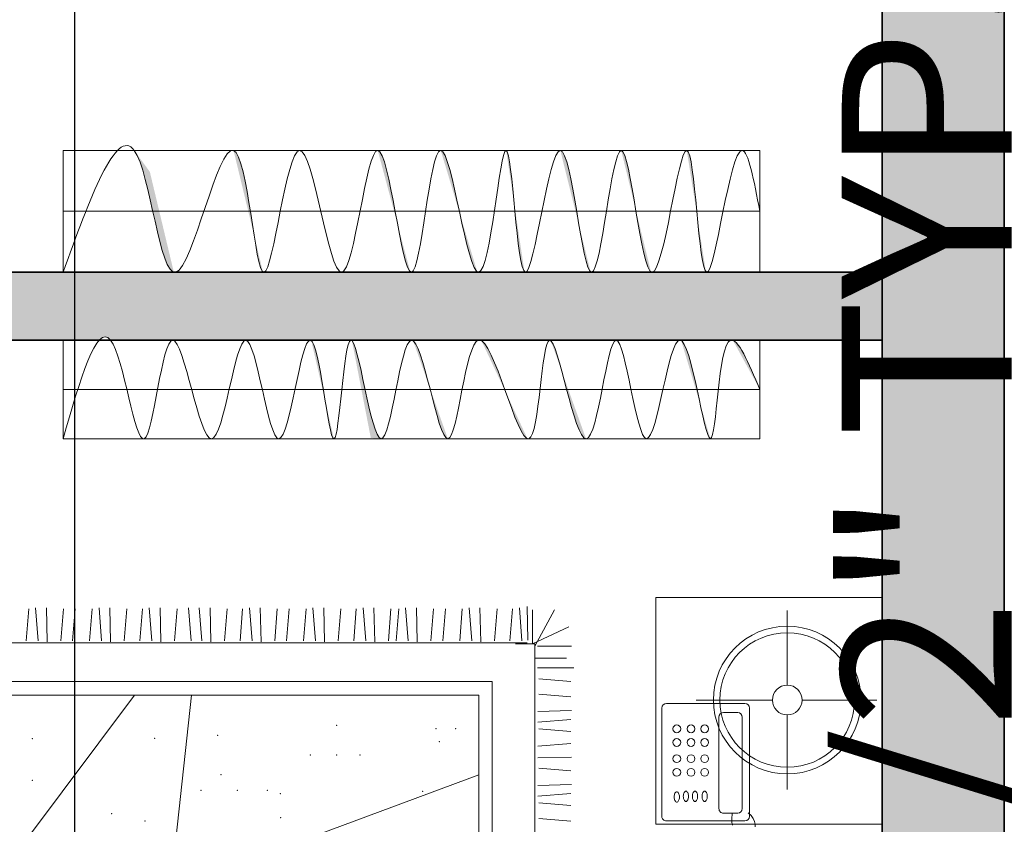
# Model space of a CAD drawing. Units: inches. Extents: x 1763 to 2368, y 1500 to 2097.
# Tile 15 of 24: x 2117 to 2189, y 1797 to 1856. Entities that reach past the tile are written whole.
import ezdxf

# ---------------------------------------------------------------- set-up
doc = ezdxf.new("R2010")
doc.units = ezdxf.units.IN
for name, color, linetype, lineweight in [('A-ANNO-DIMS', 2, 'Continuous', 18), ('A-FLOR-CASE', 8, 'Continuous', 18), ('A-FURN', 8, 'Continuous', 18), ('A-WALL', 7, 'Continuous', 35), ('A-WALL-PATT', 7, 'Continuous', 13)]:
    doc.layers.add(name, color=color, linetype=linetype, lineweight=lineweight)
doc.styles.get("Standard").update_dxf_attribs({"font": 'arial.ttf'})
doc.dimstyles.new('ISO-25', dxfattribs={"dimtxt": 12.5, "dimasz": 2.5, "dimexe": 1.25, "dimexo": 0.625, "dimtad": 1, "dimdec": 0, "dimlunit": 4, "dimtxsty": 'Standard', "dimblk": 'ARCHTICK', "dimcen": 2.5, "dimclrd": 3, "dimclrt": 4, "dimadec": 0, "dimazin": 0, "dimtfac": 1, "dimtdec": 0, "dimtmove": 0, "dimatfit": 3, "dimfxl": 1, "dimarcsym": 0})

# ---------------------------------------------------------------- blocks, each defined once
blk = doc.blocks.new('A$C77DF40FE')
for p, q in [((0.4999999828796718, 2.672344966820674), (-1.71203283e-08, 2.672344966820674)), ((-1.71203283e-08, 2.672344966820674), (-1.71203283e-08, 2.172344966820674)), ((0.4999999828796718, 2.172344966820674), (0.4999999828796718, 2.672344966820674)), ((0.2259858386969427, 2.494930331449722), (0.2259858386969427, 2.659441709452948)), ((0.0286841800407274, 2.462140050789457), (0.1931955580366775, 2.462140050789457)), ((0.2587761193572078, 2.462140050789457), (0.423287497360434, 2.462140050789457)), ((0.2259858386969427, 2.261016723758075), (0.2259858386969427, 2.429349770129192)), ((0.4937246580739157, 2.389939107844838), (0.4873052651964827, 2.38698892766115)), ((0.5000181955329026, 2.391432021402579), (0.4937246580739157, 2.389939107844838)), ((0.5060480427200674, 2.39171754290146), (0.5000181955329026, 2.391432021402579)), ((0.2337702259610523, 2.368774489841598, 10.4), (0.2337702259610523, 2.1956739737725, 10.4)), ((0.4827988465185627, 2.378774489843635, 10.4), (0.2437702259558137, 2.378774489843635, 10.4)), ((0.4808978517176002, 2.38233160625532), (0.4746402524760925, 2.375717269045708)), ((0.4873052651964827, 2.38698892766115), (0.4808978517176002, 2.38233160625532)), ((0.4927988465205999, 2.1956739737725, 10.4), (0.4927988465205999, 2.368774489841598, 10.4)), ((0.2538055232434999, 2.353040370966482, 10.4), (0.2538055232434999, 2.321546924795256, 10.4)), ((0.4656257345632185, 2.363040370968519, 10.4), (0.2638055232455372, 2.363040370968519, 10.4)), ((0.4756257345579798, 2.321546924795256, 10.4), (0.4756257345579798, 2.353040370966482, 10.4)), ((0.4766858136281372, 2.340919042260793), (0.4876185578323203, 2.34001687120326)), ((0.4876185578323203, 2.34001687120326), (0.496068234271661, 2.340226120322768)), ((0.496068234271661, 2.340226120322768), (0.5023324917128776, 2.341314910190703)), ((0.2638055232455372, 2.311546924793219, 10.4), (0.4656257345632185, 2.311546924793219, 10.4)), ((-1.71203283e-08, 2.172344966820674), (0.4999999828796718, 2.172344966820674)), ((0.2437702259558137, 2.185673973770462, 10.4), (0.4827988465185627, 2.185673973770462, 10.4)), ((0.0643996553626494, 1.980666736060811), (0.1018629931495525, 1.900293147758929)), ((0.1072148985404056, 1.9860257317996), (0.1072148985404056, 1.911011139236507)), ((0.1553804967406904, 1.991381890591583), (0.1553804967406904, 1.911011139236507)), ((0.1792009904675069, 1.913841831468744), (0.1848708171164617, 1.984665186275378)), ((0.2133772482993663, 1.913841831468744), (0.2190470749483211, 1.984665186275378)), ((0.2510109661670867, 1.911789003424928), (0.2493675302321208, 1.986512784002115)), ((0.2748401499266038, 1.911789003424928), (0.2690882152091945, 1.984870416592457)), ((0.2899179964078939, 1.913841831468744), (0.2955878230568487, 1.984665186275378)), ((0.3276571058813715, 1.911789003424928), (0.3219051711639622, 1.984870416592457)), ((0.3538856296436279, 1.911789003424928), (0.3522421937159379, 1.986512784002115)), ((0.3765634797600796, 1.913841831468744), (0.3822333064090344, 1.984665186275378)), ((0.4141971976278001, 1.911789003424928), (0.4125537617001101, 1.986512784002115)), ((0.4380263813945931, 1.911789003424928), (0.4322744466699078, 1.984870416592457)), ((0.4531042278758833, 1.913841831468744), (0.4587740545175621, 1.984665186275378)), ((0.4872804857004667, 1.913841831468744), (0.4929503123494215, 1.984665186275378)), ((0.1339744255310507, 1.975307740322023), (0.1339744255310507, 1.905652143497718)), ((0.1072148985404056, 1.905652143497718), (0.0269378679586225, 1.948518435521691)), ((0.0194810289322049, 1.888657551084179), (0.0942048095093924, 1.890300987019145)), ((0.1018629931495525, 1.900293147758929), (0.0269378679586225, 1.900293147758929)), ((0.3112043679720955, 1.905652143497718), (0.1018629931495525, 1.905652143497718)), ((0.1018629931495525, 1.905652143497718), (0.1018629931495525, 1.862788688427826)), ((0.5300974297351786, 1.905652143497718), (0.3112043679720955, 1.905652143497718)), ((0.0226663125285995, 1.871194574974651), (0.0957477256961283, 1.876946509692061)), ((0.1002397472184384, 1.888474420258717), (0.1002397472184384, 0.0935002162950696)), ((0.0247191405724152, 1.856116728493361), (0.0955424953790498, 1.850446901844406)), ((0.0247191405724152, 1.821940470661502), (0.0955424953790498, 1.816270644012547)), ((0.3112043679720955, 1.811603981208463), (0.1852251112431986, 1.811603981208463)), ((0.1852251112431986, 1.811603981208463), (0.1852251112431986, 0.1869505834038136)), ((0.5339353228555411, 1.811603981208463), (0.3112043679720955, 1.811603981208463)), ((0.0226663125285995, 1.784306752801057), (0.097390093105787, 1.785950188728747)), ((0.3112043679720955, 1.781603981209627), (0.2152251112420345, 1.781603981209627)), ((0.2152251112420345, 1.781603981209627), (0.2152251112420345, 0.2169505834026495)), ((0.5339353228555411, 1.781603981209627), (0.3112043679720955, 1.781603981209627)), ((0.3909143693745136, 1.782142099866177), (0.5339353228555411, 1.39803248996759)), ((0.0226663125285995, 1.760477569034264), (0.0957477256961283, 1.766229503751674)), ((0.0247191405724152, 1.745399722552974), (0.0955424953790498, 1.739729895904019)), ((0.0247191405724152, 1.707967178575927), (0.0955424953790498, 1.702297351926972)), ((0.0247191405724152, 1.681915979133918), (0.0955424953790498, 1.676246152484964)), ((0.0226663125285995, 1.644282261273474), (0.097390093105787, 1.645925697201164)), ((0.0226663125285995, 1.620453077506681), (0.0957477256961283, 1.62620501222409)), ((0.0247191405724152, 1.605375231025391), (0.0955424953790498, 1.599705404376436)), ((0.0247191405724152, 1.588092835292627), (0.0955424953790498, 1.582423008650948)), ((0.0226663125285995, 1.550459117432183), (0.097390093105787, 1.552102553359873)), ((0.0226663125285995, 1.52662993366539), (0.0957477256961283, 1.532381868390075)), ((0.0247191405724152, 1.511552087184099), (0.0955424953790498, 1.505882260535145)), ((0.0247191405724152, 1.47737582935224), (0.0955424953790498, 1.471706002710561)), ((0.0226663125285995, 1.439742111491796), (0.097390093105787, 1.441385547419486)), ((0.0226663125285995, 1.415912927725003), (0.0957477256961283, 1.421664862449688)), ((0.0247191405724152, 1.400835081243712), (0.0955424953790498, 1.395165254594758)), ((0.0247191405724152, 1.363402537266665), (0.0955424953790498, 1.357732710624986)), ((0.0247191405724152, 1.337351337824657), (0.0955424953790498, 1.331681511182978)), ((0.0226663125285995, 1.299717619964212), (0.097390093105787, 1.301361055891902)), ((0.0226663125285995, 1.275888436197419), (0.0957477256961283, 1.281640370922104)), ((0.0247191405724152, 1.260810589716129), (0.0955424953790498, 1.255140763067174)), ((0.0247191405724152, 1.22663433188427), (0.0955424953790498, 1.220964505242591)), ((0.0226663125285995, 1.189000614023825), (0.097390093105787, 1.190644049951515)), ((0.0226663125285995, 1.165171430257032), (0.0957477256961283, 1.170923364974441)), ((0.0226663125285995, 1.141371293764677), (0.0957477256961283, 1.147123228489363)), ((0.5339353228555411, 1.113217744226858), (0.2152251112420345, 1.147872661334986)), ((0.0247191405724152, 1.116265056378324), (0.0955424953790498, 1.110595229729369)), ((0.0226663125285995, 1.078631338510604), (0.097390093105787, 1.08027477444557)), ((0.0226663125285995, 1.054802154751087), (0.0957477256961283, 1.060554089468496)), ((0.0247191405724152, 1.039724308269796), (0.0955424953790498, 1.034054481620842)), ((0.5339353228555411, 0.783718666061759), (0.2152251112420345, 1.022135103492473)), ((0.0247191405724152, 1.005548050437937), (0.0955424953790498, 0.9998782237889827)), ((0.0226663125285995, 0.967914332570217), (0.097390093105787, 0.969557768497907)), ((0.0226663125285995, 0.944085148803424), (0.0957477256961283, 0.9498370835281092)), ((0.0247191405724152, 0.9290073023221339), (0.0955424953790498, 0.923337475680455)), ((0.0247191405724152, 0.8915747583523626), (0.0955424953790498, 0.8859049317034077)), ((0.0247191405724152, 0.865523558910354), (0.0955424953790498, 0.8598537322613992)), ((0.0226663125285995, 0.8278898410426336), (0.097390093105787, 0.8295332769775995)), ((0.0226663125285995, 0.8040606572831165), (0.0957477256961283, 0.8098125920005259)), ((0.0247191405724152, 0.7889828107945505), (0.0955424953790498, 0.7833129841528716))]:
    blk.add_line(p, q)
for centre, radius in [((0.2259858386969427, 2.462140050789457), 0.1628688693017029), ((0.2259858386969427, 2.462140050789457), 0.1484250347172038), ((0.2259858386969427, 2.462140050789457), 0.032790280659412), ((0.2895830095294514, 2.280078687035711, 10.4), 0.0085821790760856), ((0.3196359554567607, 2.280078687035711, 10.4), 0.0085821790760856), ((0.3554134417427122, 2.280078687035711, 10.4), 0.0085821790760856), ((0.3854663876700215, 2.280078687035711, 10.4), 0.0085821790760856), ((0.2895830095294514, 2.25004081246152, 10.4), 0.0085821790760856), ((0.3196359554567607, 2.25004081246152, 10.4), 0.0085821790760856), ((0.3554134417427122, 2.25004081246152, 10.4), 0.0085821790760856), ((0.3854663876700215, 2.25004081246152, 10.4), 0.0085821790760856), ((0.2895830095294514, 2.218572574704012, 10.4), 0.0085821790760856), ((0.3196359554567607, 2.218572574704012, 10.4), 0.0085821790760856), ((0.3554134417427122, 2.218572574704012, 10.4), 0.0085821790760856), ((0.3854663876700215, 2.218572574704012, 10.4), 0.0085821790760856)]:
    blk.add_circle(centre, radius)
for centre, radius, start, end in [((0.2437702259558137, 2.368774489841598, 10.4), 0.01, 90, 180), ((0.4827988465185627, 2.368774489841598, 10.4), 0.01, 0, 90), ((0.2638055232455372, 2.353040370966482, 10.4), 0.01, 90, 180), ((0.4656257345632185, 2.353040370966482, 10.4), 0.01, 0, 90), ((0.2638055232455372, 2.321546924795256, 10.4), 0.01, 180, 270), ((0.4656257345632185, 2.321546924795256, 10.4), 0.01, 270, 0), ((0.4300088254458388, 2.280078563133429, 10.4), 0.0030396816566072, 140.3607277958796, 180), ((0.4339990982480231, 2.276772912911837, 10.4), 0.0082213416638539, 116.5650513635131, 140.3607274749267), ((0.4366630074291607, 2.271445094549562, 10.4), 0.0141780236789713, 101.7009197124, 116.5650513635131), ((0.438417885095987, 2.262971795615158, 10.4), 0.0228311381682215, 90, 101.7009193040938), ((0.438417885095987, 2.262971795615158, 10.4), 0.0228311381679416, 78.29908028759999, 90), ((0.4401727627628134, 2.271445094549562, 10.4), 0.0141780236791863, 63.43494863648686, 78.29908069590611), ((0.442836671943951, 2.276772912911837, 10.4), 0.0082213416637436, 39.63927252507326, 63.43494863648686), ((0.4468269447461353, 2.280078563133429, 10.4), 0.0030396816566063, 0, 39.63927220412041), ((0.4300088254458388, 2.280078563133429, 10.4), 0.0030396816565772, 180, 219.6392725250733), ((0.4300088254458388, 2.258623115441878, 10.4), 0.0030396816566072, 140.3607277958796, 180), ((0.4339990982480231, 2.28338421335502, 10.4), 0.0082213416638406, 219.6392725250733, 243.4349486364868), ((0.4339990982480231, 2.255317465220286, 10.4), 0.0082213416638539, 116.5650513635131, 140.3607274749267), ((0.4366630074291607, 2.288712031717295, 10.4), 0.0141780236788463, 243.4349486364868, 258.2990806959061), ((0.4366630074291607, 2.249989646858011, 10.4), 0.0141780236789713, 101.7009197124, 116.5650513635131), ((0.438417885095987, 2.297185330644424, 10.4), 0.0228311381680032, 258.2990802876, 270), ((0.438417885095987, 2.241516347930883, 10.4), 0.0228311381682215, 90, 101.7009193040938), ((0.438417885095987, 2.297185330644424, 10.4), 0.022831138168207, 270, 281.7009193040939), ((0.438417885095987, 2.241516347930883, 10.4), 0.0228311381679416, 78.29908028759999, 90), ((0.4401727627628134, 2.288712031717295, 10.4), 0.014178023679087, 281.7009197124, 296.5650513635131), ((0.4401727627628134, 2.249989646858011, 10.4), 0.0141780236791863, 63.43494863648686, 78.29908069590611), ((0.442836671943951, 2.28338421335502, 10.4), 0.0082213416637319, 296.5650513635131, 320.3607274749268), ((0.442836671943951, 2.255317465220286, 10.4), 0.0082213416637436, 39.63927252507326, 63.43494863648686), ((0.4468269447461353, 2.280078563133429, 10.4), 0.0030396816565767, 320.3607274749268, 0), ((0.4468269447461353, 2.258623115441878, 10.4), 0.0030396816566063, 0, 39.63927220412041), ((0.4300088254458388, 2.258623115441878, 10.4), 0.0030396816565772, 180, 219.6392725250733), ((0.4300088254458388, 2.238597907024086, 10.4), 0.0030396816565643, 140.3607274749267, 180), ((0.4300088254458388, 2.238597907024086, 10.4), 0.0030396816565772, 180, 219.6392725250733), ((0.4339990982480231, 2.261928765663469, 10.4), 0.0082213416638406, 219.6392725250733, 243.4349486364868), ((0.4339990982480231, 2.235292256802495, 10.4), 0.0082213416638539, 116.5650513635131, 140.3607274749267), ((0.4366630074291607, 2.267256584025744, 10.4), 0.0141780236788463, 243.4349486364868, 258.2990806959061), ((0.4366630074291607, 2.229964438440219, 10.4), 0.0141780236789713, 101.7009197124, 116.5650513635131), ((0.438417885095987, 2.275729882960149, 10.4), 0.0228311381680032, 258.2990802876, 270), ((0.438417885095987, 2.221491139513091, 10.4), 0.0228311381682361, 90, 101.7009197124), ((0.438417885095987, 2.275729882960149, 10.4), 0.022831138168207, 270, 281.7009193040939), ((0.438417885095987, 2.221491139513091, 10.4), 0.0228311381679568, 78.29908028759999, 90), ((0.4401727627628134, 2.267256584025744, 10.4), 0.014178023679087, 281.7009197124, 296.5650513635131), ((0.4401727627628134, 2.229964438440219, 10.4), 0.0141780236791863, 63.43494863648686, 78.29908069590611), ((0.442836671943951, 2.261928765663469, 10.4), 0.0082213416637319, 296.5650513635131, 320.3607274749268), ((0.442836671943951, 2.235292256802495, 10.4), 0.0082213416637436, 39.63927252507326, 63.43494863648686), ((0.4468269447461353, 2.258623115441878, 10.4), 0.0030396816565767, 320.3607274749268, 0), ((0.4468269447461353, 2.238597907024086, 10.4), 0.0030396816565772, 0, 39.63927252507326), ((0.4468269447461353, 2.238597907024086, 10.4), 0.0030396816565767, 320.3607274749268, 0), ((0.4339990982480231, 2.241903557252953, 10.4), 0.0082213416638406, 219.6392725250733, 243.4349486364868), ((0.4314390647195978, 2.218572574704012, 10.4), 0.0030396816565643, 140.3607274749267, 180), ((0.4314390647195978, 2.218572574704012, 10.4), 0.0030396816565772, 180, 219.6392725250733), ((0.4354293375217822, 2.215266924482421, 10.4), 0.0082213416637416, 116.5650513635131, 140.3607274749267), ((0.4354293375217822, 2.221878224925603, 10.4), 0.0082213416637436, 219.6392725250733, 243.4349486364868), ((0.4366630074291607, 2.247231375615228, 10.4), 0.0141780236788788, 243.4349486364868, 258.2990802876), ((0.4380932467029198, 2.209939106120145, 10.4), 0.0141780236789766, 101.7009197124, 116.5650513635131), ((0.438417885095987, 2.255704674542357, 10.4), 0.0228311381679879, 258.2990806959061, 270), ((0.4398481243697461, 2.201465807193017, 10.4), 0.0228311381682215, 90, 101.7009193040938), ((0.438417885095987, 2.255704674542357, 10.4), 0.022831138168207, 270, 281.7009193040939), ((0.4398481243697461, 2.201465807193017, 10.4), 0.0228311381682253, 78.29908069590611, 90), ((0.4401727627628134, 2.247231375615228, 10.4), 0.014178023679087, 281.7009197124, 296.5650513635131), ((0.4416030020365725, 2.209939106120145, 10.4), 0.0141780236789748, 63.43494863648686, 78.29908028759999), ((0.442836671943951, 2.241903557252953, 10.4), 0.0082213416637319, 296.5650513635131, 320.3607274749268), ((0.44426691121771, 2.215266924482421, 10.4), 0.0082213416637436, 39.63927252507326, 63.43494863648686), ((0.44426691121771, 2.221878224925603, 10.4), 0.0082213416637416, 296.5650513635131, 320.3607274749268), ((0.4482571840198944, 2.218572574704012, 10.4), 0.0030396816565626, 0, 39.63927252507326), ((0.4482571840198944, 2.218572574704012, 10.4), 0.0030396816565767, 320.3607274749268, 0), ((0.2437702259558137, 2.1956739737725, 10.4), 0.01, 180, 270), ((0.4380932467029198, 2.227206043287878, 10.4), 0.0141780236788788, 243.4349486364868, 258.2990802876), ((0.4398481243697461, 2.235679342222283, 10.4), 0.0228311381679843, 258.2990806959061, 270), ((0.4398481243697461, 2.235679342222283, 10.4), 0.022831138168207, 270, 281.7009193040939), ((0.4416030020365725, 2.227206043287878, 10.4), 0.014178023679087, 281.7009197124, 296.5650513635131), ((0.4827988465185627, 2.1956739737725, 10.4), 0.01, 270, 0)]:
    blk.add_arc(centre, radius, start, end)
for p in [(0.2894910708273528, 1.731068357526964), (0.3179026300203986, 1.694587094250891), (0.2894910708273528, 1.687290920322993), (0.4274202390515712, 1.658105962196714), (0.3471074349945411, 1.519477345456834), (0.2821898240654264, 1.468403603110346), (0.3471074349945411, 1.468403603110346), (0.3471074349945411, 1.410033686843235), (0.4326481586249429, 1.344328524995944), (0.4858294848891092, 1.344367465440882), (0.4253470939220279, 1.315143435640493), (0.4253470939220279, 1.24947734545276), (0.3040933822849183, 1.205738848693727), (0.3909143693745136, 1.213035022621625), (0.4253470939220279, 1.169218644979991), (0.3106015653174836, 1.067110231953847), (0.4931307316510356, 1.04522144774819), (0.4764552750566509, 0.972219980751106), (0.3113944469878334, 0.7971491724019871), (0.4034435357025359, 0.7971102319570491)]:
    blk.add_point(p)
blk = doc.blocks.new('_ArchTick')
at = {"color": 0, "linetype": 'ByBlock', "const_width": 0.15}
blk.add_lwpolyline([(-0.5, -0.5), (0.5, 0.5)], dxfattribs=at)
blk = doc.blocks.new('*D22')
at = {"layer": 'A-ANNO-DIMS', "color": 0, "lineweight": -2, "transparency": 16777216}
for p, q in [((2189.716809557102, 2043.272690883635), (2269.316210855322, 2043.272690883635)), ((2268.066210855321, 2043.272690883635), (2268.066210855321, 1563.272690883635)), ((2189.716809557102, 1563.272690883635), (2269.316210855322, 1563.272690883635))]:
    blk.add_line(p, q, dxfattribs=at)
at = {"layer": 'Defpoints', "color": 0, "transparency": 16777216}
for p in [(2189.091809557103, 2043.272690883635), (2189.091809557103, 1563.272690883635), (2268.066210855321, 1563.272690883635)]:
    blk.add_point(p, dxfattribs=at)
at = {"layer": 'A-ANNO-DIMS', "color": 0, "lineweight": -2, "transparency": 16777216, "xscale": 2.5, "yscale": 2.5, "zscale": 2.5}
for p, rotation in [((2268.066210855321, 2043.272690883635), 90), ((2268.066210855321, 1563.272690883635), 270)]:
    blk.add_blockref('_ArchTick', p, dxfattribs=dict(at, rotation=rotation))
at = {"layer": 'A-ANNO-DIMS', "color": 0, "transparency": 16777216, "insert": (2261.059048508801, 1803.272690883634), "char_height": 12.5, "attachment_point": 5, "rotation": 90}
blk.add_mtext("40'", dxfattribs=at)
blk = doc.blocks.new('*D24')
at = {"layer": 'A-ANNO-DIMS', "color": 0, "lineweight": -2, "transparency": 16777216}
for p, q in [((2179.323431508037, 1949.352010767743), (2193.331647045969, 1949.352010767743)), ((2179.323431508037, 1862.7583987197), (2193.331647045969, 1862.7583987197))]:
    blk.add_line(p, q, dxfattribs=at)
at = {"layer": 'A-ANNO-DIMS', "color": 3, "lineweight": -2, "transparency": 16777216}
for p, q in [((2192.081647045969, 1949.352010767743), (2192.081647045969, 1862.7583987197)), ((2192.081647045969, 1862.7583987197), (2192.081647045969, 1753.790117682865))]:
    blk.add_line(p, q, dxfattribs=at)
at = {"layer": 'Defpoints', "color": 0, "transparency": 16777216}
for p in [(2178.698431508037, 1949.352010767743), (2178.698431508037, 1862.7583987197), (2192.081647045969, 1862.7583987197)]:
    blk.add_point(p, dxfattribs=at)
at = {"layer": 'A-ANNO-DIMS', "color": 3, "lineweight": -2, "transparency": 16777216, "xscale": 2.5, "yscale": 2.5, "zscale": 2.5}
for p, rotation in [((2192.081647045969, 1949.352010767743), 90), ((2192.081647045969, 1862.7583987197), 270)]:
    blk.add_blockref('_ArchTick', p, dxfattribs=dict(at, rotation=rotation))
at = {"layer": 'A-ANNO-DIMS', "color": 4, "transparency": 16777216, "insert": (2184.993481970935, 1807.024258201281), "char_height": 12.5, "attachment_point": 5, "rotation": 90}
blk.add_mtext('7\'-2 1/2" TYP.', dxfattribs=at)
blk = doc.blocks.new('*D62')
at = {"layer": 'A-ANNO-DIMS', "color": 0, "lineweight": -2, "transparency": 16777216}
for p, q in [((2083.09181, 1980.647691), (2083.09181, 1509.906119)), ((2120.612101, 1980.647691), (2120.612101, 1509.906119))]:
    blk.add_line(p, q, dxfattribs=at)
at = {"layer": 'A-ANNO-DIMS', "color": 3, "lineweight": -2, "transparency": 16777216}
for p, q in [((2083.09181, 1511.156119), (2120.612101, 1511.156119)), ((2120.612101, 1511.156119), (2186.708622145976, 1511.156119))]:
    blk.add_line(p, q, dxfattribs=at)
at = {"layer": 'Defpoints', "color": 0, "transparency": 16777216}
for p in [(2083.09181, 1981.272691), (2120.612101, 1981.272691), (2120.612101, 1511.156119)]:
    blk.add_point(p, dxfattribs=at)
at = {"layer": 'A-ANNO-DIMS', "color": 3, "lineweight": -2, "transparency": 16777216, "xscale": 2.5, "yscale": 2.5, "zscale": 2.5, "rotation": 180}
blk.add_blockref('_ArchTick', (2083.09181, 1511.156119), dxfattribs=at)
at = {"layer": 'A-ANNO-DIMS', "color": 3, "lineweight": -2, "transparency": 16777216, "xscale": 2.5, "yscale": 2.5, "zscale": 2.5}
blk.add_blockref('_ArchTick', (2120.612101, 1511.156119), dxfattribs=at)
at = {"layer": 'A-ANNO-DIMS', "color": 4, "transparency": 16777216, "insert": (2154.910361572988, 1518.248547376535), "char_height": 12.5, "attachment_point": 5}
blk.add_mtext('3\'-1 1/2"', dxfattribs=at)
blk = doc.blocks.new('*D71')
at = {"layer": 'A-ANNO-DIMS', "color": 0, "lineweight": -2, "transparency": 16777216}
for p, q in [((2049.685769, 1879.647691), (2049.685769, 1509.906119)), ((2072.784807, 1879.647691), (2072.784807, 1509.906119))]:
    blk.add_line(p, q, dxfattribs=at)
at = {"layer": 'A-ANNO-DIMS', "color": 3, "lineweight": -2, "transparency": 16777216}
for p, q in [((2049.685769, 1511.156119), (2072.784807, 1511.156119)), ((2072.784807, 1511.156119), (2118.298108500682, 1511.156119))]:
    blk.add_line(p, q, dxfattribs=at)
at = {"layer": 'Defpoints', "color": 0, "transparency": 16777216}
for p in [(2049.685769, 1880.272691), (2072.784807, 1880.272691), (2072.784807, 1511.156119)]:
    blk.add_point(p, dxfattribs=at)
at = {"layer": 'A-ANNO-DIMS', "color": 3, "lineweight": -2, "transparency": 16777216, "xscale": 2.5, "yscale": 2.5, "zscale": 2.5, "rotation": 180}
blk.add_blockref('_ArchTick', (2049.685769, 1511.156119), dxfattribs=at)
at = {"layer": 'A-ANNO-DIMS', "color": 3, "lineweight": -2, "transparency": 16777216, "xscale": 2.5, "yscale": 2.5, "zscale": 2.5}
blk.add_blockref('_ArchTick', (2072.784807, 1511.156119), dxfattribs=at)
at = {"layer": 'A-ANNO-DIMS', "color": 4, "transparency": 16777216, "insert": (2096.791457750341, 1518.056698809004), "char_height": 12.5, "attachment_point": 5}
blk.add_mtext('1\'-11"', dxfattribs=at)

msp = doc.modelspace()

# ---------------------------------------------------------------- hatches: boundary and pattern name
at = {"layer": 'A-WALL-PATT'}
h = msp.add_hatch(color=256, dxfattribs=at)
h.dxf.hatch_style = 1
h.paths.add_polyline_path([(1838.091809557101, 2034.272690883634), (1838.091809557101, 2043.272690883634), (1829.091809557101, 2043.272690883634), (1829.091809557101, 1953.387436665241), (1838.091809557101, 1953.387436665241)])
h.paths.add_polyline_path([(1838.091809557101, 1913.100906919557), (1829.091809557101, 1913.100906919557), (1829.091809557101, 1862.201751012257), (1838.091809557101, 1862.201751012257)])
h.paths.add_polyline_path([(1838.091809557101, 1825.58961200371), (1829.091809557101, 1825.58961200371), (1829.091809557101, 1738.643388462881), (1838.091809557101, 1738.643388462881)])
h.paths.add_polyline_path([(1895.591809557102, 1885.272690883634), (1838.091809557101, 1885.272690883634), (1838.091809557101, 1880.272690883634), (1895.591809557102, 1880.272690883634)])
h.paths.add_polyline_path([(1857.388795027446, 1784.272690883634), (1838.091809557101, 1784.272690883634), (1838.091809557101, 1779.272690883634), (1857.388795027446, 1779.272690883634)])
h.paths.add_polyline_path([(1958.091809557101, 1981.272690883634), (1971.455231199137, 1981.272690883634), (1971.455231199137, 1986.272690883634), (1968.567697615106, 1986.272690883634), (1958.091809557101, 1986.272690883634), (1953.091809557101, 1986.272690883634), (1927.390355781482, 1986.272690883634), (1927.390355781482, 1981.272690883634), (1953.091809557102, 1981.272690883634), (1953.091809557102, 1885.272690883634), (1932.013525308711, 1885.272690883634), (1932.013525308711, 1880.272690883634), (1959.134211901633, 1880.272690883634), (1959.134211901633, 1883.737546537067), (1959.134211901633, 1885.272690883634), (1958.091809557101, 1885.272690883634)])
h.paths.add_polyline_path([(2018.091809557102, 1981.272690883634), (2031.018823922628, 1981.272690883634), (2031.018823922628, 1986.272690883634), (2018.091809557102, 1986.272690883634), (2013.091809557101, 1986.272690883634), (2001.2328901763, 1986.272690883634), (2001.2328901763, 1981.272690883634), (2013.091809557101, 1981.272690883634), (2013.091809557101, 1885.272690883634), (1982.182180879804, 1885.272690883634, -0.0166285960272348), (1982.233249591189, 1883.737546537067), (1982.233249591189, 1880.272690883634), (2049.685769014253, 1880.272690883634), (2049.685769014253, 1883.737546537067, -0.0166285960272329), (2049.736837725638, 1885.272690883634), (2018.091809557102, 1885.272690883634)])
h.paths.add_polyline_path([(2083.091809557101, 1981.272690883633), (2120.612101449853, 1981.272690883633), (2120.612101449853, 1986.272690883634), (2083.091809557101, 1986.272690883634), (2078.091809557101, 1986.272690883634), (2063.142597715185, 1986.272690883634), (2063.142597715185, 1981.272690883634), (2078.091809557101, 1981.272690883634), (2078.091809557101, 1885.272690883634), (2072.784806703809, 1885.272690883634), (2072.784806703809, 1883.737546537067), (2072.784806703809, 1880.272690883634), (2078.091809557101, 1880.272690883634), (2078.091809557101, 1866.867159403521), (2081.556665210535, 1866.867159403521, -0.0166285960272329), (2083.091809557101, 1866.816090692136)])
h.paths.add_polyline_path([(1871.675401748104, 1635.272690883634), (1838.091809557101, 1635.272690883634), (1838.091809557101, 1626.272690883634), (1871.675401748104, 1626.272690883634)], flags=17)
h.paths.add_polyline_path([(2100.577130801176, 1688.272690883634), (2060.091809557102, 1688.272690883634), (2060.091809557102, 1679.272690883634), (2100.577130801176, 1679.272690883634)], flags=17)
h.paths.add_polyline_path([(2180.091809557101, 1688.272690883634), (2148.743529320587, 1688.272690883634), (2148.743529320587, 1679.272690883634), (2180.091809557101, 1679.272690883634)], flags=17)
h.paths.add_polyline_path([(2189.091809557101, 1746.219079973147), (2180.091809557101, 1746.219079973147), (2180.091809557101, 1743.41673524497), (2180.123283967846, 1743.41673524497), (2180.123283967846, 1726.723261858881), (2180.091809557101, 1572.272690883634), (2034.906803433656, 1572.272690883634), (2034.906803433656, 1565.600894774026), (2034.906803433656, 1563.272690883634), (2189.091809557101, 1563.272690883634)])
h.paths.add_polyline_path([(2060.091809557102, 1802.347155552507, -0.0166285960272347), (2058.556665210535, 1802.296086841122), (2055.091809557101, 1802.296086841122), (2055.091809557101, 1635.272690883634), (2042.484481853934, 1635.272690883634), (2042.484481853934, 1629.737546537067), (2042.484481853934, 1626.272690883634), (2055.091809557101, 1626.272690883634), (2055.091809557101, 1599.272690883634), (2040.268709306729, 1599.272690883634), (2040.268709306729, 1590.272690883634), (2060.091809557102, 1590.272690883634)])
h.paths.add_polyline_path([(2019.385444164378, 1629.737546537071, -0.0605692182813801), (2020.058431839583, 1635.272690883634), (1995.091809557101, 1635.272690883634), (1990.091809557101, 1635.272690883634), (1927.074869319207, 1635.272690883634), (1927.074869319207, 1626.272690883634), (1990.091809557101, 1626.272690883634), (1990.091809557102, 1590.272690883634), (1995.091809557101, 1590.272690883634), (2005.195459372391, 1590.272690883634), (2005.195459372391, 1599.272690883634), (1995.091809557101, 1599.272690883634), (1995.091809557101, 1626.272690883634), (2019.385444164378, 1626.272690883634)])
edge = h.paths.add_edge_path()
edge.add_line((2180.091809557101, 1837.272690883634), (2167.198417694339, 1837.272690883634))
edge.add_spline(control_points=[(2167.198417694823, 1837.272690883674), (2167.1907827488, 1837.271431447654), (2167.183204353112, 1837.271421440364), (2167.175683403496, 1837.272690883654)], knot_values=[168.9554928085609, 168.9554928085609, 168.9554928085609, 168.9554928085609, 169.0658706879006, 169.0658706887506, 169.0658706887506, 169.0658706887506], degree=3, periodic=0)
edge.add_spline(control_points=[(2167.175683403438, 1837.272690883663), (2166.556253545484, 1837.377242984508), (2166.326495733136, 1846.160649987724), (2165.707502931977, 1846.244137993658)], knot_values=[159.864705322856, 159.8647053237059, 159.8647053237059, 159.8647053237059, 168.9554928094108, 168.9554928094108, 168.9554928094108, 168.9554928094108], degree=3, periodic=0)
edge.add_line((2167.122451608289, 1837.272690883634), (2163.159522476786, 1837.272690883634))
edge.add_spline(control_points=[(2163.159522482475, 1837.272690883686), (2163.15796606182, 1837.2726620788), (2163.156410184994, 1837.272662044343), (2163.15485485529, 1837.272690883634)], knot_values=[150.5371721295467, 150.5371721295467, 150.5371721295467, 150.5371721295467, 150.5537966479016, 150.5537966479139, 150.5537966479139, 150.5537966479139], degree=3, periodic=0)
edge.add_spline(control_points=[(2163.154854855289, 1837.272690883634), (2162.290043487653, 1837.288726420245), (2161.594386529693, 1846.231668717186), (2160.877825059406, 1846.244137993679)], knot_values=[141.2934262950179, 141.2934262950303, 141.2934262950303, 141.2934262950303, 150.5371721295591, 150.5371721295591, 150.5371721295591, 150.5371721295591], degree=3, periodic=0)
edge.add_line((2163.075401221166, 1837.272690883634), (2158.699619590683, 1837.272690883634))
edge.add_spline(control_points=[(2158.6996195907, 1837.272690883634), (2158.698397652875, 1837.272665391618), (2158.697175755076, 1837.272665420255), (2158.695953896478, 1837.272690883674)], knot_values=[132.0335441852708, 132.0335441852708, 132.0335441852708, 132.0335441852771, 132.0491510388534, 132.0491510388534, 132.0491510388534, 132.0491510388534], degree=3, periodic=0)
edge.add_spline(control_points=[(2158.695953896478, 1837.272690883674), (2157.971966468073, 1837.287778714179), (2157.261742058153, 1846.232799164874), (2156.393385429706, 1846.244137993689)], knot_values=[122.7860209386129, 122.7860209386129, 122.7860209386129, 122.7860209386129, 132.0335441852594, 132.0335441852594, 132.0335441852594, 132.0335441852708], degree=3, periodic=0)
edge.add_line((2158.629450057908, 1837.272690883634), (2153.839354197273, 1837.272690883634))
edge.add_spline(control_points=[(2153.839354197267, 1837.272690883633), (2153.831393241206, 1837.271421595935), (2153.823483829624, 1837.271411470755), (2153.815626850732, 1837.272690883634)], knot_values=[113.4515845582001, 113.4515845582001, 113.4515845582001, 113.4515845582001, 113.5621029574639, 113.5621029574639, 113.5621029574639, 113.5621029574668], degree=3, periodic=0)
edge.add_spline(control_points=[(2153.815626850732, 1837.272690883634), (2153.16997926524, 1837.3778266931), (2152.878395890465, 1846.19087494863), (2152.403814355283, 1846.244137993689)], knot_values=[0, 0, 0, 0, 9.081854313454823, 9.081854313454823, 9.081854313454823, 9.081854313454823], degree=3, periodic=0)
edge.add_line((2153.760174359353, 1837.272690883634), (2150.390681228399, 1837.272690883634))
edge.add_spline(control_points=[(2150.390681228397, 1837.272690883634), (2150.380731407352, 1837.271531119858), (2150.370755552885, 1837.271539860845), (2150.360754310833, 1837.272690883655)], knot_values=[95.0693824194044, 95.0693824194044, 95.0693824194044, 95.06938241940794, 95.17519011295934, 95.17519011295934, 95.17519011295934, 95.17519011295934], degree=3, periodic=0)
edge.add_spline(control_points=[(2150.360754310833, 1837.272690883655), (2149.486911233016, 1837.373259724043), (2148.41925626668, 1846.194145922126), (2147.588575190972, 1846.244137993689)], knot_values=[85.8245986104526, 85.8245986104526, 85.8245986104526, 85.8245986104526, 95.06938241940442, 95.06938241940442, 95.06938241940442, 95.06938241940442], degree=3, periodic=0)
edge.add_line((2150.286144937881, 1837.272690883634), (2145.429521599744, 1837.272690883634))
edge.add_spline(control_points=[(2145.429521599744, 1837.272690883634), (2145.426173195383, 1837.272505952667), (2145.422821785984, 1837.272506511139), (2145.419467387339, 1837.272690883634)], knot_values=[76.50555885182466, 76.50555885182466, 76.50555885182466, 76.50555885182986, 76.54781121413636, 76.54781121413636, 76.54781121413636, 76.54781121413636], degree=3, periodic=0)
edge.add_spline(control_points=[(2145.419467387339, 1837.272690883634), (2144.683834601378, 1837.313124495274), (2143.804436376202, 1846.193948544996), (2142.947843667561, 1846.244137993688)], knot_values=[67.23944999382844, 67.23944999382844, 67.23944999382844, 67.23944999382844, 76.50555885179328, 76.50555885179328, 76.50555885179328, 76.50555885182465], degree=3, periodic=0)
edge.add_line((2145.353375417295, 1837.272690883634), (2134.569944747806, 1837.272690883634))
edge.add_spline(control_points=[(2134.56994474779, 1837.272690883634), (2134.566672918288, 1837.272498574207), (2134.563405957571, 1837.27249916596), (2134.560143779651, 1837.272690883636)], knot_values=[39.00146280124788, 39.00146280124788, 39.00146280124788, 39.00146280126319, 39.04510672327663, 39.04510672327663, 39.04510672327663, 39.04510672327663], degree=3, periodic=0)
edge.add_spline(control_points=[(2134.560143779651, 1837.272690883636), (2133.872211796742, 1837.313120536706), (2133.396974976361, 1845.853088067863), (2132.328029807564, 1846.244137993689)], knot_values=[29.79778030706209, 29.79778030706209, 29.79778030706209, 29.79778030706209, 39.00146280124655, 39.00146280124788, 39.00146280124788, 39.00146280124788], degree=3, periodic=0)
edge.add_line((2134.498286803723, 1837.272690883634), (2128.075271300648, 1837.272690883634))
edge.add_spline(control_points=[(2128.075271300648, 1837.272690883634), (2128.026285766884, 1837.259723584904), (2127.978195692325, 1837.26004073722), (2127.930927784897, 1837.272690883634)], knot_values=[19.48206652474599, 19.48206652474599, 19.48206652474599, 19.48206652474654, 19.86939583794397, 19.86939583794397, 19.86939583794397, 19.86939583794397], degree=3, periodic=0)
edge.add_spline(control_points=[(2125.013283184744, 1846.244137993688), (2126.164818330763, 1844.662568162717), (2126.821349600389, 1837.569643451595), (2127.930927784897, 1837.272690883634)], knot_values=[10.38980542113492, 10.3898054211352, 10.3898054211352, 10.3898054211352, 19.48206652474599, 19.48206652474599, 19.48206652474599, 19.48206652474599], degree=3, periodic=0)
edge.add_line((2127.930927784898, 1837.272690883634), (2083.091809557101, 1837.272690883634))
edge.add_line((2083.091809557101, 1837.272690883634), (2083.091809557101, 1843.768121713965))
edge.add_line((2083.091809557101, 1843.768121713965), (2081.556665210535, 1843.768121713965))
edge.add_line((2081.556665210535, 1843.768121713965), (2078.091809557101, 1843.768121713965))
edge.add_line((2078.091809557101, 1843.768121713965), (2078.091809557101, 1837.272690883634))
edge.add_line((2078.091809557101, 1837.272690883634), (2055.091809557101, 1837.272690883634))
edge.add_line((2055.091809557101, 1837.272690883634), (2055.091809557101, 1825.395124530677))
edge.add_line((2055.091809557101, 1825.395124530677), (2058.556665210535, 1825.395124530677))
edge.add_line((2058.556665210535, 1825.395124530677), (2060.091809557102, 1825.395124530677))
edge.add_line((2060.091809557102, 1825.395124530677), (2060.091809557102, 1832.272690883634))
edge.add_line((2060.091809557102, 1832.272690883634), (2122.436734598602, 1832.272690883634))
edge.add_spline(control_points=[(2122.436734598601, 1832.272690883634), (2122.727456143255, 1832.584305259818), (2123.008062474702, 1832.616792422395), (2123.275021713284, 1832.272690883634)], knot_values=[5.972032537224317, 5.972032537224317, 5.972032537224317, 5.972032537224317, 8.057258009602386, 8.057258009602837, 8.057258009602837, 8.057258009602837], degree=3, periodic=0)
edge.add_line((2123.275021713284, 1832.272690883634), (2137.951393308032, 1832.272690883634))
edge.add_spline(control_points=[(2137.951393307966, 1832.272690883629), (2137.961042543445, 1832.274026104781), (2137.970676309981, 1832.27403826157), (2137.980294423909, 1832.272690883634)], knot_values=[53.92686179676418, 53.92686179676418, 53.92686179676418, 53.92686179676418, 54.03007548000314, 54.03007548000314, 54.03007548000314, 54.03007548000601], degree=3, periodic=0)
edge.add_spline(control_points=[(2139.715582741171, 1825.016325920323), (2139.281482802356, 1825.062086475526), (2138.671282749905, 1832.175892027703), (2137.98029442391, 1832.272690883634)], knot_values=[54.03007548000314, 54.03007548000314, 54.03007548000314, 54.03007548000314, 61.44519353062353, 61.44519353062641, 61.44519353062641, 61.44519353062641], degree=3, periodic=0)
edge.add_line((2138.045183132032, 1832.272690883634), (2140.961787078569, 1832.272690883634))
edge.add_spline(control_points=[(2140.96178707854, 1832.272690883628), (2140.970606368947, 1832.274440590632), (2140.979501539198, 1832.27442261757), (2140.988470957723, 1832.272690883634)], knot_values=[68.85418231261454, 68.85418231261454, 68.85418231261454, 68.85418231280003, 68.97123731673409, 68.97123731673409, 68.97123731673409, 68.97123731673409], degree=3, periodic=0)
edge.add_spline(control_points=[(2143.18986511145, 1825.016325920314), (2142.436495288906, 1825.065396856983), (2141.561146249046, 1832.16212393513), (2140.988470957723, 1832.272690883634)], knot_values=[68.9712373167341, 68.97123731708082, 68.97123731708082, 68.97123731708082, 76.44491114487315, 76.44491114487315, 76.44491114487315, 76.44491114487315], degree=3, periodic=0)
edge.add_line((2141.040932085754, 1832.272690883634), (2145.429521599744, 1832.272690883634))
edge.add_spline(control_points=[(2145.429521599742, 1832.272690883634), (2145.43886220747, 1832.273579662711), (2145.448227241903, 1832.27357314134), (2145.457616067813, 1832.272690883634)], knot_values=[84.03904662338796, 84.03904662338796, 84.03904662338796, 84.03904662338971, 84.12404068496751, 84.12404068496751, 84.12404068496751, 84.12404068496751], degree=3, periodic=0)
edge.add_spline(control_points=[(2148.107765738118, 1825.016325920317), (2147.340420200817, 1825.019697773855), (2146.30265295, 1832.193283691691), (2145.457616067813, 1832.272690883634)], knot_values=[84.12404068496751, 84.12404068496751, 84.12404068496751, 84.12404068496751, 91.77389142141917, 91.77389142141917, 91.77389142141917, 91.77389142141917], degree=3, periodic=0)
edge.add_line((2145.537886823607, 1832.272690883634), (2150.392945902062, 1832.272690883634))
edge.add_spline(control_points=[(2150.392945902064, 1832.272690883634), (2150.41883348599, 1832.27702102203), (2150.445058688081, 1832.276951395392), (2150.471602715227, 1832.272690883634)], knot_values=[99.38157707204087, 99.3815770720414, 99.3815770720414, 99.3815770720414, 99.57345662964875, 99.57345662964875, 99.57345662964875, 99.57345662964875], degree=3, periodic=0)
edge.add_spline(control_points=[(2153.974048108825, 1825.016325920308), (2153.092849423049, 1825.280585632922), (2151.529174697084, 1832.102942795321), (2150.471602715227, 1832.272690883634)], knot_values=[99.57345662964875, 99.57345662964875, 99.57345662964875, 99.57345662964875, 107.2183570397887, 107.2183570397887, 107.2183570397887, 107.2183570397887], degree=3, periodic=0)
edge.add_line((2150.568426065927, 1832.272690883634), (2155.598049458685, 1832.272690883634))
edge.add_spline(control_points=[(2155.59804945868, 1832.272690883633), (2155.604650662926, 1832.273493563234), (2155.611310013868, 1832.273487964753), (2155.618026602473, 1832.272690883629)], knot_values=[114.9330576886776, 114.9330576886776, 114.9330576886776, 114.9330576886986, 115.0136243763172, 115.0136243763172, 115.0136243763172, 115.0136243763172], degree=3, periodic=0)
edge.add_spline(control_points=[(2158.284655371249, 1825.016325920309), (2157.395326401988, 1825.074357796858), (2156.251834921329, 1832.197474627747), (2155.618026602473, 1832.272690883629)], knot_values=[115.0136243763171, 115.0136243763171, 115.0136243763171, 115.0136243763171, 122.6162690869638, 122.6162690869638, 122.6162690869638, 122.6162690869638], degree=3, periodic=0)
edge.add_line((2155.677997005666, 1832.272690883634), (2165.194843181567, 1832.272690883634))
edge.add_spline(control_points=[(2165.194843180774, 1832.272690883621), (2165.197973141718, 1832.272787704364), (2165.201103815629, 1832.272787940576), (2165.204235204227, 1832.27269088363)], knot_values=[145.4884769441583, 145.4884769441583, 145.4884769441583, 145.4884769441583, 145.5163785292906, 145.5163785298517, 145.5163785298517, 145.5163785298517], degree=3, periodic=0)
edge.add_spline(control_points=[(2167.445935353137, 1825.016325920312), (2166.960552374007, 1825.022023955429), (2166.055957046383, 1832.246291885329), (2165.204235204289, 1832.272690883628)], knot_values=[145.5163785292906, 145.5163785292906, 145.5163785292906, 145.5163785292906, 153.1054685509886, 153.1054685509886, 153.1054685509886, 153.1054685515498], degree=3, periodic=0)
edge.add_line((2165.289510410991, 1832.272690883634), (2168.928217296476, 1832.272690883634))
edge.add_spline(control_points=[(2168.928217296468, 1832.272690883631), (2168.9815111362, 1832.293215999779), (2169.037604970232, 1832.292507987016), (2169.096218703475, 1832.272690883634)], knot_values=[160.5174393135676, 160.5174393135676, 160.5174393135676, 160.5174393135912, 160.9397230621378, 160.9397230621378, 160.9397230621378, 160.9397230621378], degree=3, periodic=0)
edge.add_spline(control_points=[(2171.08610288907, 1828.644508401971), (2170.354822507508, 1830.369456517115), (2169.623542125945, 1832.094404632258), (2169.096218703475, 1832.272690883634)], knot_values=[160.9397230621378, 160.9397230621378, 160.9397230621378, 160.9397230621378, 164.7388346221332, 164.7388346221332, 164.7388346221332, 164.7388346221332], degree=3, periodic=0)
edge.add_line((2169.096218703475, 1832.272690883634), (2180.091809557101, 1832.272690883634))
edge.add_line((2180.091809557101, 1832.272690883634), (2180.091809557101, 1837.272690883634))
h.paths.add_polyline_path([(2189.091809557101, 1885.522968548043), (2180.091809557101, 1885.522968548043), (2180.091809557101, 1813.316873906924), (2180.123283967846, 1813.316873906924), (2180.123283967846, 1796.623400520835), (2180.123092181994, 1795.256344207559), (2189.091809557101, 1795.256344207559)])
h.paths.add_polyline_path([(2180.091809557101, 1986.272690883634), (2166.279557011185, 1986.272690883634), (2166.279557011185, 1981.272690883634), (2180.091809557101, 1981.272690883634)])
h.paths.add_polyline_path([(2189.091809557101, 2043.272690883634), (2180.091809557101, 2043.272690883634), (2180.091809557101, 2034.272690883634), (2180.091809557101, 1934.108443350786), (2189.091809557101, 1934.108443350786)])
h.paths.add_polyline_path([(1838.091809557101, 1681.591873076235), (1829.091809557101, 1681.591873076235), (1829.091809557101, 1563.272690883634), (2003.864084895099, 1563.272690883634), (2003.864084895099, 1565.600894774026), (2003.864084895099, 1572.272690883634), (1838.091809557101, 1572.272690883634)])

# ---------------------------------------------------------------- linework, layer by layer
at = {"layer": 'A-FLOR-CASE'}
for p, q in [((2119.772940310415, 1841.758414438661), (2171.08610288907, 1841.758414438661)), ((2119.772940310415, 1828.644508401971), (2171.08610288907, 1828.644508401971))]:
    msp.add_line(p, q, dxfattribs=at)
for points in [[(2119.772940310415, 1846.244137993689), (2171.08610288907, 1846.244137993689), (2171.08610288907, 1837.272690883634), (2119.772940310415, 1837.272690883634)], [(2119.772940310415, 1832.272690883634), (2171.08610288907, 1832.272690883634), (2171.08610288907, 1825.016325920308), (2119.772940310415, 1825.016325920308)]]:
    msp.add_lwpolyline(points, close=True, dxfattribs=at)
for points, knots in [([(2119.772940310415, 1837.272690883634), (2121.73517716088, 1842.662051202745), (2125.487746061776, 1852.968628578668), (2127.570267147068, 1828.953763057942), (2132.892423798528, 1855.105326932265), (2134.356527079077, 1828.518958683748), (2137.132722428043, 1855.227137572787), (2140.387218981168, 1828.254843406616), (2142.919962416673, 1855.204859980233), (2145.56738814461, 1828.351118599332), (2147.34748062016, 1855.247214515429), (2150.572117006053, 1828.246460091184), (2152.583194607929, 1855.11327373109), (2153.469672077686, 1828.319672331732), (2156.546577474337, 1855.277089424158), (2158.683081495254, 1828.313103925907), (2160.897955290289, 1855.200051722259), (2162.990561550039, 1828.252180094126), (2166.090754481521, 1855.172797783424), (2166.792330596212, 1828.352257930181), (2169.384242572585, 1850.750864662884), (2170.660520126767, 1844.007148820224), (2171.08610288907, 1841.758414438661)], [0, 0, 0, 0, 10.38980542113492, 19.86939583794342, 29.79778030706341, 39.04510672326133, 48.39295608004983, 57.87980892633894, 67.23944999382846, 76.54781121413114, 85.77210362691523, 95.1751901129558, 104.3697302447449, 113.4515845582001, 122.7860209386129, 132.0491510388471, 141.2805315996552, 150.537172129559, 159.8647053217126, 168.9554928094108, 178.2963125081795, 182.9693067330485, 182.9693067330485, 182.9693067330485, 182.9693067330485]), ([(2119.772940310415, 1825.016325920308), (2121.008219169356, 1829.309308184063), (2123.419114121483, 1837.6879258495), (2125.839204930159, 1818.385740092247), (2127.653625415973, 1839.377274481216), (2130.83424025712, 1817.734364298319), (2133.212076931808, 1839.524750190017), (2135.676816228946, 1817.730877379582), (2138.049588364897, 1839.527702610493), (2139.894591848377, 1817.863101683683), (2140.669640662759, 1839.484788907215), (2143.316095076274, 1817.742890625), (2145.246367580785, 1839.553998016228), (2148.366929742155, 1817.806463346518), (2149.896697540325, 1839.682129213062), (2154.749265331607, 1817.685452803815), (2155.110705345501, 1839.427115066769), (2158.552059596111, 1817.719144196201), (2160.437750373757, 1839.488146760734), (2162.739710121653, 1817.747880819909), (2165.143511811743, 1839.543991900488), (2167.84479006573, 1817.955115108844), (2168.035416609379, 1835.840483681392), (2170.273538287267, 1830.561190175), (2171.08610288907, 1828.644508401971)], [0, 0, 0, 0, 8.057258009602386, 15.72535830492602, 23.2796926104922, 31.07824447751822, 38.76002787005681, 46.41464719194286, 54.03007548000601, 61.49299643082029, 68.85418231280003, 76.44491114487313, 84.03904662338971, 91.77389142835565, 99.38157707204087, 107.5184973541071, 114.9330576886986, 122.6783785679101, 130.2610702792425, 137.8561476627419, 145.5163785292906, 153.1114559127895, 160.5174393135912, 164.7388346221332, 164.7388346221332, 164.7388346221332, 164.7388346221332])]:
    msp.add_open_spline(points, degree=3, knots=knots, dxfattribs=at)
at = {"layer": 'A-WALL'}
for p, q in [((2180.091809557101, 2034.272690883634), (2180.091809557101, 1572.272690883634)), ((2083.091809557101, 1837.272690883634), (2180.091809557101, 1837.272690883634)), ((2060.091809557102, 1832.272690883634), (2180.091809557101, 1832.272690883634))]:
    msp.add_line(p, q, dxfattribs=at)
msp.add_lwpolyline([(2003.864084895099, 1563.272690883634), (1829.091809557101, 1563.272690883634), (1829.091809557101, 2043.272690883634), (2189.091809557101, 2043.272690883634), (2189.091809557101, 1563.272690883634), (2034.906803433656, 1563.272690883634)], dxfattribs=at)

# ---------------------------------------------------------------- block references
at = {"layer": 'A-FURN', "xscale": 33.38694677217886, "yscale": 33.38694677217886, "zscale": 33.38694677217886, "rotation": 270}
msp.add_blockref('A$C77DF40FE', (2090.901844803704, 1813.316873335329), dxfattribs=at)

# ---------------------------------------------------------------- dimensions: what is measured, and where the dimension line sits
at = {"layer": 'A-ANNO-DIMS'}
dim = msp.add_linear_dim(base=(2268.066210855321, 1563.272690883635), p1=(2189.091809557101, 2043.272690883634), p2=(2189.091809557101, 1563.272690883634), angle=90, dimstyle='ISO-25', override={"dimclrd": 0, "dimclre": 0, "dimclrt": 0}, dxfattribs=at)
dim.commit()
dim.dimension.update_dxf_attribs({"geometry": '*D22', "text_midpoint": (2261.059048508801, 1803.272690883634)})
for base, p1, p2, picture, middle in [((2120.612101, 1511.156119), (2083.09181, 1981.272691), (2120.612101, 1981.272691), '*D62', (2154.910361572988, 1518.248547376535)), ((2072.784807, 1511.156119), (2049.685769, 1880.272691), (2072.784807, 1880.272691), '*D71', (2096.791457750341, 1518.056698809004))]:
    dim = msp.add_linear_dim(base=base, p1=p1, p2=p2, dimstyle='ISO-25', override={"dimdec": 1, "dimlfac": 1, "dimrnd": 0, "dimzin": 1, "dimdsep": 46, "dimlunit": 4, "dimfrac": 2}, dxfattribs=at)
    dim.commit()
    dim.dimension.update_dxf_attribs({"geometry": picture, "text_midpoint": middle})
dim = msp.add_linear_dim(base=(2192.081647045969, 1862.7583987197), p1=(2178.698431508036, 1949.352010767742), p2=(2178.698431508036, 1862.758398719699), angle=270, text='<> TYP.', dimstyle='ISO-25', override={"dimdec": 1, "dimlfac": 1, "dimrnd": 0, "dimzin": 1, "dimdsep": 46, "dimlunit": 4, "dimfrac": 2}, dxfattribs=at)
dim.commit()
dim.dimension.update_dxf_attribs({"geometry": '*D24', "text_midpoint": (2184.993481970935, 1807.024258201281)})

doc.saveas('drawing.dxf')
